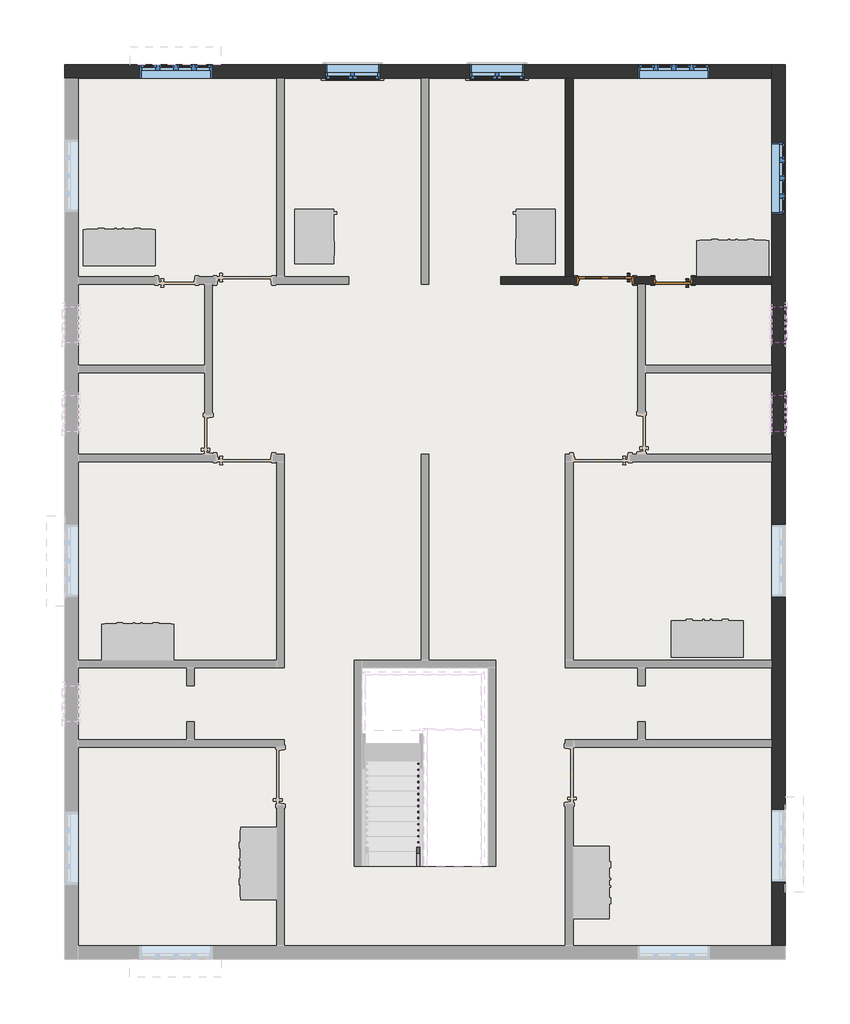
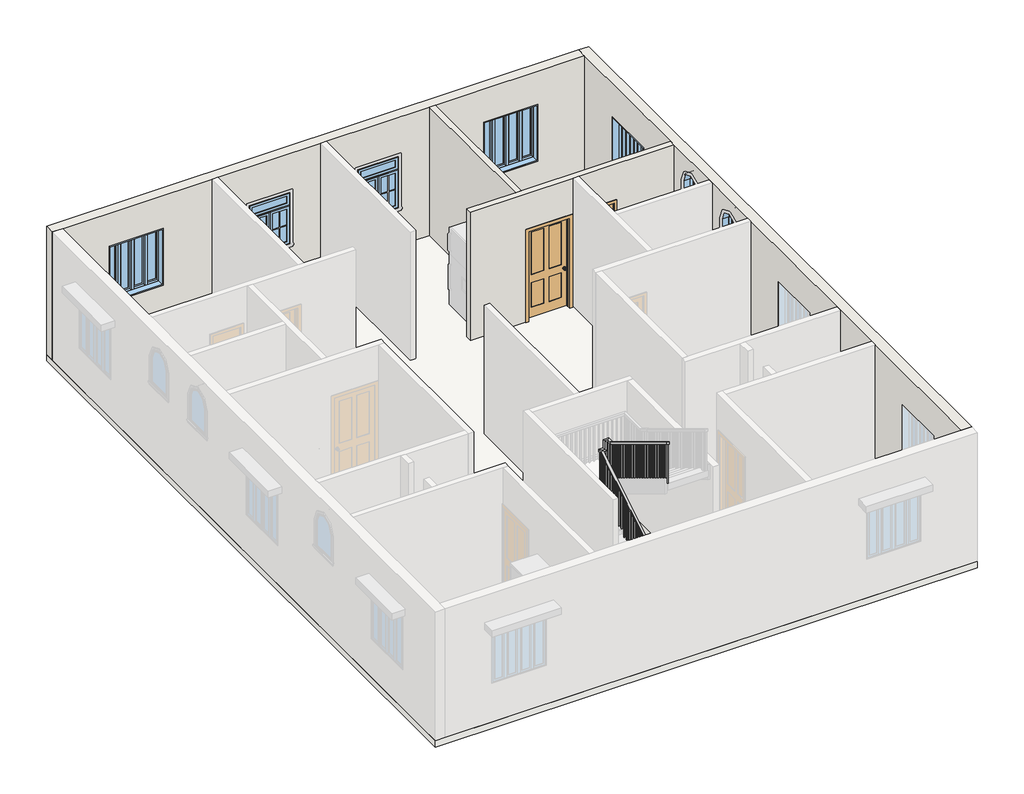
# One storey, part 2 of 4: 7 windows, 4 walls, 2 doors, 1 railing, 1 slab.
"""IFC4 building model written with IfcOpenShell, lengths in millimetres."""

from ifc_helpers import new_model, si_unit, frame, origin, place, context, project, spatial, polyline, circle_curve, outline, extrude, faceted_brep, transform, mapped, element, save
from ifc_brep_helpers import plane_surface, revolved_surface, advanced_brep
from components import door_a823658d, door_3f5f64ee, window_casement_double_transom_0fae6a54, window_casement_multi_sash_horizontal_main_windows_4_x_7_0e27d311, window_2fd4accf

model = new_model("IFC4")

# Units and contexts
model_context = context("Model", 3, world=origin())
ifc_project = project(units=[si_unit("LENGTHUNIT", "METRE", prefix="MILLI")], contexts=[model_context])

# Site, building, storey
site = spatial("IfcSite", under=ifc_project)
building = spatial("IfcBuilding", under=site)
storey = spatial("IfcBuildingStorey", under=building, Elevation=3352.8)

# Doors
placement = place(None, origin())
door_shape = door_a823658d(model_context)
element("IfcDoor", 1, ObjectType="Door-Interior-Single-4_Panel-Wood : 36\" x 84\"", at=placement, inside=storey, context=model_context, shape_type="MappedRepresentation", body=[
    mapped(door_shape, transform((-6490.9771954, 4939.0022103, 3352.8), x_axis=(-1.0, 0.0, 0.0), y_axis=(0.0, -1.0, 0.0), z_axis=(0.0, 0.0, 1.0))),
])
door_2_shape = door_3f5f64ee(model_context)
element("IfcDoor", 2, ObjectType="Door-Interior-Single-Flush_Panel-Wood : 24\" x 84\"", at=placement, inside=storey, context=model_context, shape_type="MappedRepresentation", body=[
    mapped(door_2_shape, transform((-5347.9771954, 4932.6522103, 3352.8), x_axis=(-1.0, 0.0, 0.0), y_axis=(0.0, -1.0, 0.0), z_axis=(0.0, 0.0, 1.0))),
])

# Railing
element("IfcRailing", 3, ObjectType="Handrail - Rectangular", at=placement, inside=storey, context=model_context, shape_type="SolidModel", body=[
    faceted_brep([(-9678.6771954, -4957.4727897, 4419.6), (-9678.6771954, -4957.4727897, 4360.3575287), (-9627.8771954, -4957.4727897, 4360.3575287), (-9627.8771954, -4957.4727897, 4419.6), (-9678.6771954, -2671.4727897, 5791.2), (-9678.6771954, -2657.4020042, 5740.4), (-9627.8771954, -2657.4020042, 5740.4), (-9627.8771954, -2671.4727897, 5791.2), (-9678.6771954, -2588.9227897, 5791.2), (-9678.6771954, -2588.9227897, 5740.4), (-9627.8771954, -2639.7227897, 5740.4), (-9627.8771954, -2639.7227897, 5791.2), (-9577.0771954, -2588.9227897, 5791.2), (-9526.2771954, -2588.9227897, 5740.4), (-9526.2771954, -2639.7227897, 5740.4), (-9577.0771954, -2639.7227897, 5791.2), (-9577.0771954, -2588.9227897, 5989.32), (-9526.2771954, -2588.9227897, 5938.52), (-9526.2771954, -2639.7227897, 5938.52), (-9577.0771954, -2639.7227897, 5989.32), (-9450.0771954, -2588.9227897, 5989.32), (-9450.0771954, -2588.9227897, 5938.52), (-9500.8771954, -2639.7227897, 5938.52), (-9500.8771954, -2639.7227897, 5989.32), (-9450.0771954, -2715.9227897, 5989.32), (-9450.0771954, -2729.9935751, 5938.52), (-9500.8771954, -2729.9935751, 5938.52), (-9500.8771954, -2715.9227897, 5989.32), (-9450.0771954, -4925.7227897, 7315.2), (-9500.8771954, -4925.7227897, 7315.2), (-9500.8771954, -4925.7227897, 7255.9575287), (-9450.0771954, -4925.7227897, 7255.9575287)], [[[0, 1, 2, 3]], [[1, 0, 4, 5]], [[2, 1, 5, 6]], [[3, 2, 6, 7]], [[0, 3, 7, 4]], [[5, 4, 8, 9]], [[6, 5, 9, 10]], [[7, 6, 10, 11]], [[4, 7, 11, 8]], [[9, 8, 12, 13]], [[10, 9, 13, 14]], [[11, 10, 14, 15]], [[8, 11, 15, 12]], [[13, 12, 16, 17]], [[14, 13, 17, 18]], [[15, 14, 18, 19]], [[12, 15, 19, 16]], [[17, 16, 20, 21]], [[18, 17, 21, 22]], [[19, 18, 22, 23]], [[16, 19, 23, 20]], [[21, 20, 24, 25]], [[22, 21, 25, 26]], [[23, 22, 26, 27]], [[20, 23, 27, 24]], [[28, 29, 30, 31]], [[25, 24, 28, 31]], [[26, 25, 31, 30]], [[27, 26, 30, 29]], [[24, 27, 29, 28]]]),
    extrude(outline(polyline([(-4859.0477897, 7215.9525287), (-4839.9977897, 7204.5225287), (-4839.9977897, 6248.4), (-4859.0477897, 6248.4), (-4859.0477897, 7215.9525287)])), frame((-9485.0021954, 0.0, 0.0), z_axis=(1.0, 0.0, 0.0), x_axis=(0.0, 1.0, 0.0)), (0.0, 0.0, 1.0), 19.05),
    extrude(outline(polyline([(-4757.4477897, 7154.9925287), (-4738.3977897, 7143.5625287), (-4738.3977897, 6248.4), (-4757.4477897, 6248.4), (-4757.4477897, 7154.9925287)])), frame((-9485.0021954, 0.0, 0.0), z_axis=(1.0, 0.0, 0.0), x_axis=(0.0, 1.0, 0.0)), (0.0, 0.0, 1.0), 19.05),
    extrude(outline(polyline([(-4655.8477897, 7094.0325287), (-4636.7977897, 7082.6025287), (-4636.7977897, 6096.0), (-4655.8477897, 6096.0), (-4655.8477897, 7094.0325287)])), frame((-9485.0021954, 0.0, 0.0), z_axis=(1.0, 0.0, 0.0), x_axis=(0.0, 1.0, 0.0)), (0.0, 0.0, 1.0), 19.05),
    extrude(outline(polyline([(-4554.2477897, 7033.0725287), (-4535.1977897, 7021.6425287), (-4535.1977897, 6096.0), (-4554.2477897, 6096.0), (-4554.2477897, 7033.0725287)])), frame((-9485.0021954, 0.0, 0.0), z_axis=(1.0, 0.0, 0.0), x_axis=(0.0, 1.0, 0.0)), (0.0, 0.0, 1.0), 19.05),
    extrude(outline(polyline([(-4452.6477897, 6972.1125287), (-4433.5977897, 6960.6825287), (-4433.5977897, 6096.0), (-4452.6477897, 6096.0), (-4452.6477897, 6972.1125287)])), frame((-9485.0021954, 0.0, 0.0), z_axis=(1.0, 0.0, 0.0), x_axis=(0.0, 1.0, 0.0)), (0.0, 0.0, 1.0), 19.05),
    extrude(outline(polyline([(-4351.0477897, 6911.1525287), (-4331.9977897, 6899.7225287), (-4331.9977897, 5943.6), (-4351.0477897, 5943.6), (-4351.0477897, 6911.1525287)])), frame((-9485.0021954, 0.0, 0.0), z_axis=(1.0, 0.0, 0.0), x_axis=(0.0, 1.0, 0.0)), (0.0, 0.0, 1.0), 19.05),
    extrude(outline(polyline([(-4249.4477897, 6850.1925287), (-4230.3977897, 6838.7625287), (-4230.3977897, 5943.6), (-4249.4477897, 5943.6), (-4249.4477897, 6850.1925287)])), frame((-9485.0021954, 0.0, 0.0), z_axis=(1.0, 0.0, 0.0), x_axis=(0.0, 1.0, 0.0)), (0.0, 0.0, 1.0), 19.05),
    extrude(outline(polyline([(-4147.8477897, 6789.2325287), (-4128.7977897, 6777.8025287), (-4128.7977897, 5791.2), (-4147.8477897, 5791.2), (-4147.8477897, 6789.2325287)])), frame((-9485.0021954, 0.0, 0.0), z_axis=(1.0, 0.0, 0.0), x_axis=(0.0, 1.0, 0.0)), (0.0, 0.0, 1.0), 19.05),
    extrude(outline(polyline([(-4046.2477897, 6728.2725287), (-4027.1977897, 6716.8425287), (-4027.1977897, 5791.2), (-4046.2477897, 5791.2), (-4046.2477897, 6728.2725287)])), frame((-9485.0021954, 0.0, 0.0), z_axis=(1.0, 0.0, 0.0), x_axis=(0.0, 1.0, 0.0)), (0.0, 0.0, 1.0), 19.05),
    extrude(outline(polyline([(-3944.6477897, 6667.3125287), (-3925.5977897, 6655.8825287), (-3925.5977897, 5791.2), (-3944.6477897, 5791.2), (-3944.6477897, 6667.3125287)])), frame((-9485.0021954, 0.0, 0.0), z_axis=(1.0, 0.0, 0.0), x_axis=(0.0, 1.0, 0.0)), (0.0, 0.0, 1.0), 19.05),
    extrude(outline(polyline([(-3843.0477897, 6606.3525287), (-3823.9977897, 6594.9225287), (-3823.9977897, 5638.8), (-3843.0477897, 5638.8), (-3843.0477897, 6606.3525287)])), frame((-9485.0021954, 0.0, 0.0), z_axis=(1.0, 0.0, 0.0), x_axis=(0.0, 1.0, 0.0)), (0.0, 0.0, 1.0), 19.05),
    extrude(outline(polyline([(-3741.4477897, 6545.3925287), (-3722.3977897, 6533.9625287), (-3722.3977897, 5638.8), (-3741.4477897, 5638.8), (-3741.4477897, 6545.3925287)])), frame((-9485.0021954, 0.0, 0.0), z_axis=(1.0, 0.0, 0.0), x_axis=(0.0, 1.0, 0.0)), (0.0, 0.0, 1.0), 19.05),
    extrude(outline(polyline([(-3639.8477897, 6484.4325287), (-3620.7977897, 6473.0025287), (-3620.7977897, 5486.4), (-3639.8477897, 5486.4), (-3639.8477897, 6484.4325287)])), frame((-9485.0021954, 0.0, 0.0), z_axis=(1.0, 0.0, 0.0), x_axis=(0.0, 1.0, 0.0)), (0.0, 0.0, 1.0), 19.05),
    extrude(outline(polyline([(-3538.2477897, 6423.4725287), (-3519.1977897, 6412.0425287), (-3519.1977897, 5486.4), (-3538.2477897, 5486.4), (-3538.2477897, 6423.4725287)])), frame((-9485.0021954, 0.0, 0.0), z_axis=(1.0, 0.0, 0.0), x_axis=(0.0, 1.0, 0.0)), (0.0, 0.0, 1.0), 19.05),
    extrude(outline(polyline([(-3436.6477897, 6362.5125287), (-3417.5977897, 6351.0825287), (-3417.5977897, 5486.4), (-3436.6477897, 5486.4), (-3436.6477897, 6362.5125287)])), frame((-9485.0021954, 0.0, 0.0), z_axis=(1.0, 0.0, 0.0), x_axis=(0.0, 1.0, 0.0)), (0.0, 0.0, 1.0), 19.05),
    extrude(outline(polyline([(-3335.0477897, 6301.5525287), (-3315.9977897, 6290.1225287), (-3315.9977897, 5334.0), (-3335.0477897, 5334.0), (-3335.0477897, 6301.5525287)])), frame((-9485.0021954, 0.0, 0.0), z_axis=(1.0, 0.0, 0.0), x_axis=(0.0, 1.0, 0.0)), (0.0, 0.0, 1.0), 19.05),
    extrude(outline(polyline([(-3233.4477897, 6240.5925287), (-3214.3977897, 6229.1625287), (-3214.3977897, 5334.0), (-3233.4477897, 5334.0), (-3233.4477897, 6240.5925287)])), frame((-9485.0021954, 0.0, 0.0), z_axis=(1.0, 0.0, 0.0), x_axis=(0.0, 1.0, 0.0)), (0.0, 0.0, 1.0), 19.05),
    extrude(outline(polyline([(-3131.8477897, 6179.6325287), (-3112.7977897, 6168.2025287), (-3112.7977897, 5181.6), (-3131.8477897, 5181.6), (-3131.8477897, 6179.6325287)])), frame((-9485.0021954, 0.0, 0.0), z_axis=(1.0, 0.0, 0.0), x_axis=(0.0, 1.0, 0.0)), (0.0, 0.0, 1.0), 19.05),
    extrude(outline(polyline([(-3030.2477897, 6118.6725287), (-3011.1977897, 6107.2425287), (-3011.1977897, 5181.6), (-3030.2477897, 5181.6), (-3030.2477897, 6118.6725287)])), frame((-9485.0021954, 0.0, 0.0), z_axis=(1.0, 0.0, 0.0), x_axis=(0.0, 1.0, 0.0)), (0.0, 0.0, 1.0), 19.05),
    extrude(outline(polyline([(-2928.6477897, 6057.7125287), (-2909.5977897, 6046.2825287), (-2909.5977897, 5181.6), (-2928.6477897, 5181.6), (-2928.6477897, 6057.7125287)])), frame((-9485.0021954, 0.0, 0.0), z_axis=(1.0, 0.0, 0.0), x_axis=(0.0, 1.0, 0.0)), (0.0, 0.0, 1.0), 19.05),
    extrude(outline(polyline([(-2827.0477897, 5996.7525287), (-2807.9977897, 5985.3225287), (-2807.9977897, 5029.2), (-2827.0477897, 5029.2), (-2827.0477897, 5996.7525287)])), frame((-9485.0021954, 0.0, 0.0), z_axis=(1.0, 0.0, 0.0), x_axis=(0.0, 1.0, 0.0)), (0.0, 0.0, 1.0), 19.05),
    extrude(outline(polyline([(-2725.4477897, 5935.7925287), (-2706.3977897, 5924.3625287), (-2706.3977897, 5029.2), (-2725.4477897, 5029.2), (-2725.4477897, 5935.7925287)])), frame((-9485.0021954, 0.0, 0.0), z_axis=(1.0, 0.0, 0.0), x_axis=(0.0, 1.0, 0.0)), (0.0, 0.0, 1.0), 19.05),
    extrude(outline(polyline([(-9561.2021954, -2623.8477897), (-9561.2021954, -2604.7977897), (-9542.1521954, -2604.7977897), (-9542.1521954, -2623.8477897), (-9561.2021954, -2623.8477897)])), frame((0.0, 0.0, 4876.8), z_axis=(0.0, 0.0, 1.0), x_axis=(1.0, 0.0, 0.0)), (0.0, 0.0, 1.0), 1061.72),
    extrude(outline(polyline([(-2731.7977897, 5695.7625287), (-2712.7477897, 5707.1925287), (-2712.7477897, 4724.4), (-2731.7977897, 4724.4), (-2731.7977897, 5695.7625287)])), frame((-9662.8021954, 0.0, 0.0), z_axis=(1.0, 0.0, 0.0), x_axis=(0.0, 1.0, 0.0)), (0.0, 0.0, 1.0), 19.05),
    extrude(outline(polyline([(-2833.3977897, 5634.8025287), (-2814.3477897, 5646.2325287), (-2814.3477897, 4724.4), (-2833.3977897, 4724.4), (-2833.3977897, 5634.8025287)])), frame((-9662.8021954, 0.0, 0.0), z_axis=(1.0, 0.0, 0.0), x_axis=(0.0, 1.0, 0.0)), (0.0, 0.0, 1.0), 19.05),
    extrude(outline(polyline([(-2934.9977897, 5573.8425287), (-2915.9477897, 5585.2725287), (-2915.9477897, 4724.4), (-2934.9977897, 4724.4), (-2934.9977897, 5573.8425287)])), frame((-9662.8021954, 0.0, 0.0), z_axis=(1.0, 0.0, 0.0), x_axis=(0.0, 1.0, 0.0)), (0.0, 0.0, 1.0), 19.05),
    extrude(outline(polyline([(-3036.5977897, 5512.8825287), (-3017.5477897, 5524.3125287), (-3017.5477897, 4572.0), (-3036.5977897, 4572.0), (-3036.5977897, 5512.8825287)])), frame((-9662.8021954, 0.0, 0.0), z_axis=(1.0, 0.0, 0.0), x_axis=(0.0, 1.0, 0.0)), (0.0, 0.0, 1.0), 19.05),
    extrude(outline(polyline([(-3138.1977897, 5451.9225287), (-3119.1477897, 5463.3525287), (-3119.1477897, 4572.0), (-3138.1977897, 4572.0), (-3138.1977897, 5451.9225287)])), frame((-9662.8021954, 0.0, 0.0), z_axis=(1.0, 0.0, 0.0), x_axis=(0.0, 1.0, 0.0)), (0.0, 0.0, 1.0), 19.05),
    extrude(outline(polyline([(-3239.7977897, 5390.9625287), (-3220.7477897, 5402.3925287), (-3220.7477897, 4419.6), (-3239.7977897, 4419.6), (-3239.7977897, 5390.9625287)])), frame((-9662.8021954, 0.0, 0.0), z_axis=(1.0, 0.0, 0.0), x_axis=(0.0, 1.0, 0.0)), (0.0, 0.0, 1.0), 19.05),
    extrude(outline(polyline([(-3341.3977897, 5330.0025287), (-3322.3477897, 5341.4325287), (-3322.3477897, 4419.6), (-3341.3977897, 4419.6), (-3341.3977897, 5330.0025287)])), frame((-9662.8021954, 0.0, 0.0), z_axis=(1.0, 0.0, 0.0), x_axis=(0.0, 1.0, 0.0)), (0.0, 0.0, 1.0), 19.05),
    extrude(outline(polyline([(-3442.9977897, 5269.0425287), (-3423.9477897, 5280.4725287), (-3423.9477897, 4419.6), (-3442.9977897, 4419.6), (-3442.9977897, 5269.0425287)])), frame((-9662.8021954, 0.0, 0.0), z_axis=(1.0, 0.0, 0.0), x_axis=(0.0, 1.0, 0.0)), (0.0, 0.0, 1.0), 19.05),
    extrude(outline(polyline([(-3544.5977897, 5208.0825287), (-3525.5477897, 5219.5125287), (-3525.5477897, 4267.2), (-3544.5977897, 4267.2), (-3544.5977897, 5208.0825287)])), frame((-9662.8021954, 0.0, 0.0), z_axis=(1.0, 0.0, 0.0), x_axis=(0.0, 1.0, 0.0)), (0.0, 0.0, 1.0), 19.05),
    extrude(outline(polyline([(-3646.1977897, 5147.1225287), (-3627.1477897, 5158.5525287), (-3627.1477897, 4267.2), (-3646.1977897, 4267.2), (-3646.1977897, 5147.1225287)])), frame((-9662.8021954, 0.0, 0.0), z_axis=(1.0, 0.0, 0.0), x_axis=(0.0, 1.0, 0.0)), (0.0, 0.0, 1.0), 19.05),
    extrude(outline(polyline([(-3747.7977897, 5086.1625287), (-3728.7477897, 5097.5925287), (-3728.7477897, 4114.8), (-3747.7977897, 4114.8), (-3747.7977897, 5086.1625287)])), frame((-9662.8021954, 0.0, 0.0), z_axis=(1.0, 0.0, 0.0), x_axis=(0.0, 1.0, 0.0)), (0.0, 0.0, 1.0), 19.05),
    extrude(outline(polyline([(-3849.3977897, 5025.2025287), (-3830.3477897, 5036.6325287), (-3830.3477897, 4114.8), (-3849.3977897, 4114.8), (-3849.3977897, 5025.2025287)])), frame((-9662.8021954, 0.0, 0.0), z_axis=(1.0, 0.0, 0.0), x_axis=(0.0, 1.0, 0.0)), (0.0, 0.0, 1.0), 19.05),
    extrude(outline(polyline([(-3950.9977897, 4964.2425287), (-3931.9477897, 4975.6725287), (-3931.9477897, 4114.8), (-3950.9977897, 4114.8), (-3950.9977897, 4964.2425287)])), frame((-9662.8021954, 0.0, 0.0), z_axis=(1.0, 0.0, 0.0), x_axis=(0.0, 1.0, 0.0)), (0.0, 0.0, 1.0), 19.05),
    extrude(outline(polyline([(-4052.5977897, 4903.2825287), (-4033.5477897, 4914.7125287), (-4033.5477897, 3962.4), (-4052.5977897, 3962.4), (-4052.5977897, 4903.2825287)])), frame((-9662.8021954, 0.0, 0.0), z_axis=(1.0, 0.0, 0.0), x_axis=(0.0, 1.0, 0.0)), (0.0, 0.0, 1.0), 19.05),
    extrude(outline(polyline([(-4154.1977897, 4842.3225287), (-4135.1477897, 4853.7525287), (-4135.1477897, 3962.4), (-4154.1977897, 3962.4), (-4154.1977897, 4842.3225287)])), frame((-9662.8021954, 0.0, 0.0), z_axis=(1.0, 0.0, 0.0), x_axis=(0.0, 1.0, 0.0)), (0.0, 0.0, 1.0), 19.05),
    extrude(outline(polyline([(-4255.7977897, 4781.3625287), (-4236.7477897, 4792.7925287), (-4236.7477897, 3810.0), (-4255.7977897, 3810.0), (-4255.7977897, 4781.3625287)])), frame((-9662.8021954, 0.0, 0.0), z_axis=(1.0, 0.0, 0.0), x_axis=(0.0, 1.0, 0.0)), (0.0, 0.0, 1.0), 19.05),
    extrude(outline(polyline([(-4357.3977897, 4720.4025287), (-4338.3477897, 4731.8325287), (-4338.3477897, 3810.0), (-4357.3977897, 3810.0), (-4357.3977897, 4720.4025287)])), frame((-9662.8021954, 0.0, 0.0), z_axis=(1.0, 0.0, 0.0), x_axis=(0.0, 1.0, 0.0)), (0.0, 0.0, 1.0), 19.05),
    extrude(outline(polyline([(-4458.9977897, 4659.4425287), (-4439.9477897, 4670.8725287), (-4439.9477897, 3810.0), (-4458.9977897, 3810.0), (-4458.9977897, 4659.4425287)])), frame((-9662.8021954, 0.0, 0.0), z_axis=(1.0, 0.0, 0.0), x_axis=(0.0, 1.0, 0.0)), (0.0, 0.0, 1.0), 19.05),
    extrude(outline(polyline([(-4560.5977897, 4598.4825287), (-4541.5477897, 4609.9125287), (-4541.5477897, 3657.6), (-4560.5977897, 3657.6), (-4560.5977897, 4598.4825287)])), frame((-9662.8021954, 0.0, 0.0), z_axis=(1.0, 0.0, 0.0), x_axis=(0.0, 1.0, 0.0)), (0.0, 0.0, 1.0), 19.05),
    extrude(outline(polyline([(-4662.1977897, 4537.5225287), (-4643.1477897, 4548.9525287), (-4643.1477897, 3657.6), (-4662.1977897, 3657.6), (-4662.1977897, 4537.5225287)])), frame((-9662.8021954, 0.0, 0.0), z_axis=(1.0, 0.0, 0.0), x_axis=(0.0, 1.0, 0.0)), (0.0, 0.0, 1.0), 19.05),
    extrude(outline(polyline([(-4763.7977897, 4476.5625287), (-4744.7477897, 4487.9925287), (-4744.7477897, 3505.2), (-4763.7977897, 3505.2), (-4763.7977897, 4476.5625287)])), frame((-9662.8021954, 0.0, 0.0), z_axis=(1.0, 0.0, 0.0), x_axis=(0.0, 1.0, 0.0)), (0.0, 0.0, 1.0), 19.05),
    extrude(outline(polyline([(-4865.3977897, 4415.6025287), (-4846.3477897, 4427.0325287), (-4846.3477897, 3505.2), (-4865.3977897, 3505.2), (-4865.3977897, 4415.6025287)])), frame((-9662.8021954, 0.0, 0.0), z_axis=(1.0, 0.0, 0.0), x_axis=(0.0, 1.0, 0.0)), (0.0, 0.0, 1.0), 19.05),
    extrude(outline(polyline([(-9485.0021954, -2623.8477897), (-9485.0021954, -2604.7977897), (-9465.9521954, -2604.7977897), (-9465.9521954, -2623.8477897), (-9485.0021954, -2623.8477897)])), frame((0.0, 0.0, 4876.8), z_axis=(0.0, 0.0, 1.0), x_axis=(1.0, 0.0, 0.0)), (0.0, 0.0, 1.0), 1061.72),
    extrude(outline(polyline([(-9643.7521954, -2623.8477897), (-9662.8021954, -2623.8477897), (-9662.8021954, -2604.7977897), (-9643.7521954, -2604.7977897), (-9643.7521954, -2623.8477897)])), frame((0.0, 0.0, 4876.8), z_axis=(0.0, 0.0, 1.0), x_axis=(1.0, 0.0, 0.0)), (0.0, 0.0, 1.0), 863.6),
    extrude(outline(polyline([(-2680.9977897, 5726.2425287), (-2661.9477897, 5737.6725287), (-2661.9477897, 4876.8), (-2680.9977897, 4876.8), (-2680.9977897, 5726.2425287)])), frame((-9662.8021954, 0.0, 0.0), z_axis=(1.0, 0.0, 0.0), x_axis=(0.0, 1.0, 0.0)), (0.0, 0.0, 1.0), 19.05),
    extrude(outline(polyline([(-4925.7227897, 7255.9575287), (-4906.6727897, 7244.5275287), (-4906.6727897, 6248.4), (-4925.7227897, 6248.4), (-4925.7227897, 7255.9575287)])), frame((-9485.0021954, 0.0, 0.0), z_axis=(1.0, 0.0, 0.0), x_axis=(0.0, 1.0, 0.0)), (0.0, 0.0, 1.0), 19.05),
    extrude(outline(polyline([(-4957.4727897, 4360.3575287), (-4938.4227897, 4371.7875287), (-4938.4227897, 3505.2), (-4957.4727897, 3505.2), (-4957.4727897, 4360.3575287)])), frame((-9662.8021954, 0.0, 0.0), z_axis=(1.0, 0.0, 0.0), x_axis=(0.0, 1.0, 0.0)), (0.0, 0.0, 1.0), 19.05),
])

# Slab
element("IfcSlab", 4, ObjectType="MARBLE FLOORING 6\"", at=placement, inside=storey, context=model_context, shape_type="SweptSolid", body=[
    extrude(outline(polyline([(-3455.6771954, 8580.7272103), (-3455.6771954, -6532.2727897), (-15623.8646954, -6532.2727897), (-15623.8646954, 8580.7272103), (-3455.6771954, 8580.7272103)]), holes=[polyline([(-10605.7771954, -4957.4727897), (-8472.1771954, -4957.4727897), (-8472.1771954, -1604.6727897), (-10605.7771954, -1604.6727897), (-10605.7771954, -4957.4727897)])]), frame((0.0, 0.0, 3200.4), z_axis=(0.0, 0.0, 1.0), x_axis=(1.0, 0.0, 0.0)), (0.0, 0.0, 1.0), 152.4),
])

# Walls
element("IfcWall", 5, ObjectType="INNER WALL 5\"", at=placement, inside=storey, context=model_context, shape_type="Brep", body=[
    faceted_brep([(-3684.2771954, 4872.3272103, 6400.8), (-5817.8771954, 4872.3272103, 6400.8), (-5944.8771954, 4872.3272103, 6400.8), (-8256.2771954, 4872.3272103, 6400.8), (-8256.2771954, 4872.3272103, 3352.8), (-6973.5771954, 4872.3272103, 3352.8), (-6973.5771954, 4872.3272103, 5511.8), (-6008.3771954, 4872.3272103, 5511.8), (-6008.3771954, 4872.3272103, 3352.8), (-5944.8771954, 4872.3272103, 3352.8), (-5817.8771954, 4872.3272103, 3352.8), (-5678.1771954, 4872.3272103, 3352.8), (-5678.1771954, 4872.3272103, 5511.8), (-5017.7771954, 4872.3272103, 5511.8), (-5017.7771954, 4872.3272103, 3352.8), (-3684.2771954, 4872.3272103, 3352.8), (-8256.2771954, 4999.3272103, 6400.8), (-7164.0771954, 4999.3272103, 6400.8), (-7037.0771954, 4999.3272103, 6400.8), (-3684.2771954, 4999.3272103, 6400.8), (-3684.2771954, 4999.3272103, 3352.8), (-5017.7771954, 4999.3272103, 3352.8), (-5017.7771954, 4999.3272103, 5511.8), (-5678.1771954, 4999.3272103, 5511.8), (-5678.1771954, 4999.3272103, 3352.8), (-6008.3771954, 4999.3272103, 3352.8), (-6008.3771954, 4999.3272103, 5511.8), (-6973.5771954, 4999.3272103, 5511.8), (-6973.5771954, 4999.3272103, 3352.8), (-7037.0771954, 4999.3272103, 3352.8), (-7164.0771954, 4999.3272103, 3352.8), (-8256.2771954, 4999.3272103, 3352.8)], [[[0, 1, 2, 3, 4, 5, 6, 7, 8, 9, 10, 11, 12, 13, 14, 15]], [[16, 17, 18, 19, 20, 21, 22, 23, 24, 25, 26, 27, 28, 29, 30, 31]], [[4, 31, 30, 29, 28, 5]], [[20, 15, 14, 21]], [[8, 25, 24, 11, 10, 9]], [[3, 2, 1, 0, 19, 18, 17, 16]], [[4, 3, 16, 31]], [[0, 15, 20, 19]], [[27, 6, 5, 28]], [[6, 27, 26, 7]], [[7, 26, 25, 8]], [[23, 12, 11, 24]], [[12, 23, 22, 13]], [[13, 22, 21, 14]]]),
])
element("IfcWall", 6, ObjectType="INNER WALL 5\"", at=placement, inside=storey, context=model_context, shape_type="SweptSolid", body=[
    extrude(outline(polyline([(-7164.0771954, 4999.3272103), (-7164.0771954, 8352.1272103), (-7037.0771954, 8352.1272103), (-7037.0771954, 4999.3272103), (-7164.0771954, 4999.3272103)])), frame((0.0, 0.0, 3352.8), z_axis=(0.0, 0.0, 1.0), x_axis=(1.0, 0.0, 0.0)), (0.0, 0.0, 1.0), 3048.0),
])
element("IfcWall", 7, ObjectType="OUTER WALL 9\"", at=placement, inside=storey, context=model_context, shape_type="Brep", body=[
    faceted_brep([(-15623.8646954, 8352.1272103, 3352.8), (-15395.2646954, 8352.1272103, 3352.8), (-12040.8771954, 8352.1272103, 3352.8), (-11913.8771954, 8352.1272103, 3352.8), (-9602.4771954, 8352.1272103, 3352.8), (-9475.4771954, 8352.1272103, 3352.8), (-7164.0771954, 8352.1272103, 3352.8), (-7037.0771954, 8352.1272103, 3352.8), (-3684.2771954, 8352.1272103, 3352.8), (-3684.2771954, 8352.1272103, 6400.8), (-7037.0771954, 8352.1272103, 6400.8), (-7164.0771954, 8352.1272103, 6400.8), (-9475.4771954, 8352.1272103, 6400.8), (-9602.4771954, 8352.1272103, 6400.8), (-11913.8771954, 8352.1272103, 6400.8), (-12040.8771954, 8352.1272103, 6400.8), (-15395.2646954, 8352.1272103, 6400.8), (-15623.8646954, 8352.1272103, 6400.8), (-13133.8709454, 8352.1272103, 5613.4), (-13133.8709454, 8352.1272103, 4267.2), (-14353.0709454, 8352.1272103, 4267.2), (-14353.0709454, 8352.1272103, 5613.4), (-4725.6771954, 8352.1272103, 5613.4), (-4725.6771954, 8352.1272103, 4267.2), (-5944.8771954, 8352.1272103, 4267.2), (-5944.8771954, 8352.1272103, 5613.4), (-10300.9771954, 8352.1272103, 5486.4), (-10300.9771954, 8352.1272103, 4267.2), (-11215.3771954, 8352.1272103, 4267.2), (-11215.3771954, 8352.1272103, 5486.4), (-7862.5771954, 8352.1272103, 5486.4), (-7862.5771954, 8352.1272103, 4267.2), (-8776.9771954, 8352.1272103, 4267.2), (-8776.9771954, 8352.1272103, 5486.4), (-15623.8646954, 8580.7272103, 3352.8), (-15623.8646954, 8580.7272103, 6400.8), (-3684.2771954, 8580.7272103, 6400.8), (-3684.2771954, 8580.7272103, 3352.8), (-13133.8709454, 8580.7272103, 5613.4), (-14353.0709454, 8580.7272103, 5613.4), (-14353.0709454, 8580.7272103, 4267.2), (-13133.8709454, 8580.7272103, 4267.2), (-4725.6771954, 8580.7272103, 5613.4), (-5944.8771954, 8580.7272103, 5613.4), (-5944.8771954, 8580.7272103, 4267.2), (-4725.6771954, 8580.7272103, 4267.2), (-10300.9771954, 8580.7272103, 5486.4), (-11215.3771954, 8580.7272103, 5486.4), (-11215.3771954, 8580.7272103, 4267.2), (-10300.9771954, 8580.7272103, 4267.2), (-7862.5771954, 8580.7272103, 5486.4), (-8776.9771954, 8580.7272103, 5486.4), (-8776.9771954, 8580.7272103, 4267.2), (-7862.5771954, 8580.7272103, 4267.2)], [[[0, 1, 2, 3, 4, 5, 6, 7, 8, 9, 10, 11, 12, 13, 14, 15, 16, 17], [18, 19, 20, 21], [22, 23, 24, 25], [26, 27, 28, 29], [30, 31, 32, 33]], [[34, 35, 36, 37], [38, 39, 40, 41], [42, 43, 44, 45], [46, 47, 48, 49], [50, 51, 52, 53]], [[8, 7, 6, 5, 4, 3, 2, 1, 0, 34, 37]], [[17, 16, 15, 14, 13, 12, 11, 10, 9, 36, 35]], [[0, 17, 35, 34]], [[9, 8, 37, 36]], [[19, 18, 38, 41]], [[20, 19, 41, 40]], [[21, 20, 40, 39]], [[18, 21, 39, 38]], [[23, 22, 42, 45]], [[24, 23, 45, 44]], [[25, 24, 44, 43]], [[22, 25, 43, 42]], [[27, 26, 46, 49]], [[28, 27, 49, 48]], [[29, 28, 48, 47]], [[26, 29, 47, 46]], [[31, 30, 50, 53]], [[32, 31, 53, 52]], [[33, 32, 52, 51]], [[30, 33, 51, 50]]]),
])
element("IfcWall", 8, ObjectType="OUTER WALL 9\"", at=placement, inside=storey, context=model_context, shape_type="AdvancedBrep", body=[
    advanced_brep(
    [(-3684.2771954, 8580.7272103, 3352.8), (-3684.2771954, 8352.1272103, 3352.8), (-3684.2771954, 4999.3272103, 3352.8), (-3684.2771954, 4872.3272103, 3352.8), (-3684.2771954, 3500.7272103, 3352.8), (-3684.2771954, 3373.7272103, 3352.8), (-3684.2771954, 2002.6566069, 3352.8), (-3684.2771954, 1875.6566069, 3352.8), (-3684.2771954, -1477.6727897, 3352.8), (-3684.2771954, -1604.6727897, 3352.8), (-3684.2771954, -2823.8727897, 3352.8), (-3684.2771954, -2950.8727897, 3352.8), (-3684.2771954, -6303.6727897, 3352.8), (-3684.2771954, -6303.6727897, 6400.8), (-3684.2771954, -2950.8727897, 6400.8), (-3684.2771954, -2823.8727897, 6400.8), (-3684.2771954, -1604.6727897, 6400.8), (-3684.2771954, -1477.6727897, 6400.8), (-3684.2771954, 1875.6566069, 6400.8), (-3684.2771954, 2002.6566069, 6400.8), (-3684.2771954, 3373.7272103, 6400.8), (-3684.2771954, 3500.7272103, 6400.8), (-3684.2771954, 4872.3272103, 6400.8), (-3684.2771954, 4999.3272103, 6400.8), (-3684.2771954, 8352.1272103, 6400.8), (-3684.2771954, 8580.7272103, 6400.8), (-3684.2771954, 6053.4272103, 5613.4), (-3684.2771954, 6053.4272103, 4267.2), (-3684.2771954, 7272.6272103, 4267.2), (-3684.2771954, 7272.6272103, 5613.4), (-3684.2771954, -410.6080914, 5613.4), (-3684.2771954, -410.6080914, 4267.2), (-3684.2771954, 808.5919086, 4267.2), (-3684.2771954, 808.5919086, 5613.4), (-3684.2771954, -4004.9727897, 5613.4), (-3684.2771954, -5224.1727897, 5613.4), (-3684.2771954, -5224.1727897, 4267.2), (-3684.2771954, -4004.9727897, 4267.2), (-3684.2771954, 2992.9919086, 5181.6), (-3684.2771954, 2992.9919086, 5791.2), (-3684.2771954, 2383.3919086, 5791.2), (-3684.2771954, 2383.3919086, 5181.6), (-3684.2771954, 4491.3272103, 5181.6), (-3684.2771954, 4491.3272103, 5791.2), (-3684.2771954, 3881.7272103, 5791.2), (-3684.2771954, 3881.7272103, 5181.6), (-3455.6771954, 8580.7272103, 3352.8), (-3455.6771954, 8580.7272103, 6400.8), (-3455.6771954, -6303.6727897, 6400.8), (-3455.6771954, -6303.6727897, 3352.8), (-3455.6771954, 6053.4272103, 5613.4), (-3455.6771954, 7272.6272103, 5613.4), (-3455.6771954, 7272.6272103, 4267.2), (-3455.6771954, 6053.4272103, 4267.2), (-3455.6771954, -410.6080914, 5613.4), (-3455.6771954, 808.5919086, 5613.4), (-3455.6771954, 808.5919086, 4267.2), (-3455.6771954, -410.6080914, 4267.2), (-3455.6771954, -4004.9727897, 5613.4), (-3455.6771954, -4004.9727897, 4267.2), (-3455.6771954, -5224.1727897, 4267.2), (-3455.6771954, -5224.1727897, 5613.4), (-3455.6771954, 2992.9919086, 5181.6), (-3455.6771954, 2383.3919086, 5181.6), (-3455.6771954, 2383.3919086, 5791.2), (-3455.6771954, 2992.9919086, 5791.2), (-3455.6771954, 4491.3272103, 5181.6), (-3455.6771954, 3881.7272103, 5181.6), (-3455.6771954, 3881.7272103, 5791.2), (-3455.6771954, 4491.3272103, 5791.2)],
    [
        (0, 1),
        (1, 2),
        (2, 3),
        (3, 4),
        (4, 5),
        (5, 6),
        (6, 7),
        (7, 8),
        (8, 9),
        (9, 10),
        (10, 11),
        (11, 12),
        (12, 13),
        (13, 14),
        (14, 15),
        (15, 16),
        (16, 17),
        (17, 18),
        (18, 19),
        (19, 20),
        (20, 21),
        (21, 22),
        (22, 23),
        (23, 24),
        (24, 25),
        (25, 0),
        (26, 27),
        (27, 28),
        (28, 29),
        (29, 26),
        (30, 31),
        (31, 32),
        (32, 33),
        (33, 30),
        (34, 35),
        (35, 36),
        (36, 37),
        (37, 34),
        (38, 39),
        (39, 40, circle_curve(frame((-3684.2771954, 2688.1919086, 5791.2), z_axis=(1.0, 0.0, 0.0), x_axis=(0.0, -1.0, 0.0)), 304.8)),
        (40, 41),
        (41, 38),
        (42, 43),
        (43, 44, circle_curve(frame((-3684.2771954, 4186.5272103, 5791.2), z_axis=(1.0, 0.0, 0.0), x_axis=(0.0, -1.0, 0.0)), 304.8)),
        (44, 45),
        (45, 42),
        (46, 47),
        (47, 48),
        (48, 49),
        (49, 46),
        (50, 51),
        (51, 52),
        (52, 53),
        (53, 50),
        (54, 55),
        (55, 56),
        (56, 57),
        (57, 54),
        (58, 59),
        (59, 60),
        (60, 61),
        (61, 58),
        (62, 63),
        (63, 64),
        (64, 65, circle_curve(frame((-3455.6771954, 2688.1919086, 5791.2), z_axis=(-1.0, 0.0, 0.0), x_axis=(0.0, -1.0, 0.0)), 304.8)),
        (65, 62),
        (66, 67),
        (67, 68),
        (68, 69, circle_curve(frame((-3455.6771954, 4186.5272103, 5791.2), z_axis=(-1.0, 0.0, 0.0), x_axis=(0.0, -1.0, 0.0)), 304.8)),
        (69, 66),
        (0, 46),
        (49, 12),
        (13, 48),
        (47, 25),
        (26, 50),
        (53, 27),
        (52, 28),
        (51, 29),
        (30, 54),
        (57, 31),
        (56, 32),
        (55, 33),
        (58, 34),
        (37, 59),
        (36, 60),
        (35, 61),
        (62, 38),
        (41, 63),
        (40, 64),
        (39, 65),
        (66, 42),
        (45, 67),
        (44, 68),
        (43, 69),
    ],
    [
        plane_surface(frame((-3684.2771954, 8466.4272103, 3352.8), z_axis=(-1.0, 0.0, 0.0), x_axis=(0.0, -1.0, 0.0))),
        plane_surface(frame((-3455.6771954, 8466.4272103, 3352.8), z_axis=(1.0, 0.0, 0.0), x_axis=(0.0, 1.0, 0.0))),
        plane_surface(frame((-3684.2771954, 8466.4272103, 3352.8), z_axis=(0.0, 0.0, -1.0), x_axis=(1.0, 0.0, 0.0))),
        plane_surface(frame((-3684.2771954, -6417.9727897, 6400.8), z_axis=(0.0, 0.0, 1.0), x_axis=(1.0, 0.0, 0.0))),
        plane_surface(frame((-15509.5646954, 8580.7272103, 3352.8), z_axis=(0.0, 1.0, 0.0), x_axis=(-1.0, 0.0, 0.0))),
        plane_surface(frame((-3569.9771954, -6303.6727897, 3352.8), z_axis=(0.0, -1.0, 0.0), x_axis=(-1.0, 0.0, 0.0))),
        plane_surface(frame((-3684.2771954, 6053.4272103, 5613.4), z_axis=(0.0, 1.0, 0.0), x_axis=(1.0, 0.0, 0.0))),
        plane_surface(frame((-3684.2771954, 6053.4272103, 4267.2), z_axis=(0.0, 0.0, 1.0), x_axis=(1.0, 0.0, 0.0))),
        plane_surface(frame((-3684.2771954, 7272.6272103, 4267.2), z_axis=(0.0, -1.0, 0.0), x_axis=(1.0, 0.0, 0.0))),
        plane_surface(frame((-3684.2771954, 7272.6272103, 5613.4), z_axis=(0.0, 0.0, -1.0), x_axis=(1.0, 0.0, 0.0))),
        plane_surface(frame((-3684.2771954, -410.6080914, 5613.4), z_axis=(0.0, 1.0, 0.0), x_axis=(1.0, 0.0, 0.0))),
        plane_surface(frame((-3684.2771954, -410.6080914, 4267.2), z_axis=(0.0, 0.0, 1.0), x_axis=(1.0, 0.0, 0.0))),
        plane_surface(frame((-3684.2771954, 808.5919086, 4267.2), z_axis=(0.0, -1.0, 0.0), x_axis=(1.0, 0.0, 0.0))),
        plane_surface(frame((-3684.2771954, 808.5919086, 5613.4), z_axis=(0.0, 0.0, -1.0), x_axis=(1.0, 0.0, 0.0))),
        plane_surface(frame((-3455.6771954, -4004.9727897, 5613.4), z_axis=(0.0, -1.0, 0.0), x_axis=(-1.0, 0.0, 0.0))),
        plane_surface(frame((-3455.6771954, -4004.9727897, 4267.2), z_axis=(0.0, 0.0, 1.0), x_axis=(-1.0, 0.0, 0.0))),
        plane_surface(frame((-3455.6771954, -5224.1727897, 4267.2), z_axis=(0.0, 1.0, 0.0), x_axis=(-1.0, 0.0, 0.0))),
        plane_surface(frame((-3455.6771954, -5224.1727897, 5613.4), z_axis=(0.0, 0.0, -1.0), x_axis=(-1.0, 0.0, 0.0))),
        plane_surface(frame((-3455.6771954, 2992.9919086, 5181.6), z_axis=(0.0, 0.0, 1.0), x_axis=(-1.0, 0.0, 0.0))),
        plane_surface(frame((-3455.6771954, 2383.3919086, 5181.6), z_axis=(0.0, 1.0, 0.0), x_axis=(-1.0, 0.0, 0.0))),
        revolved_surface(polyline([(-3684.2771954, 2383.3919085999996, 5791.2), (-3455.6771954, 2383.3919085999996, 5791.2)]), (-3684.2771954, 2688.1919086, 5791.2), (-1.0, 0.0, 0.0)),
        plane_surface(frame((-3455.6771954, 2992.9919086, 5791.2), z_axis=(0.0, -1.0, 0.0), x_axis=(-1.0, 0.0, 0.0))),
        plane_surface(frame((-3455.6771954, 4491.3272103, 5181.6), z_axis=(0.0, 0.0, 1.0), x_axis=(-1.0, 0.0, 0.0))),
        plane_surface(frame((-3455.6771954, 3881.7272103, 5181.6), z_axis=(0.0, 1.0, 0.0), x_axis=(-1.0, 0.0, 0.0))),
        revolved_surface(polyline([(-3684.2771954, 3881.7272102999996, 5791.2), (-3455.6771954, 3881.7272102999996, 5791.2)]), (-3684.2771954, 4186.5272103, 5791.2), (-1.0, 0.0, 0.0)),
        plane_surface(frame((-3455.6771954, 4491.3272103, 5791.2), z_axis=(0.0, -1.0, 0.0), x_axis=(-1.0, 0.0, 0.0))),
    ],
    [
        (0, [[1, 2, 3, 4, 5, 6, 7, 8, 9, 10, 11, 12, 13, 14, 15, 16, 17, 18, 19, 20, 21, 22, 23, 24, 25, 26], [27, 28, 29, 30], [31, 32, 33, 34], [35, 36, 37, 38], [39, 40, 41, 42], [43, 44, 45, 46]]),
        (1, [[47, 48, 49, 50], [51, 52, 53, 54], [55, 56, 57, 58], [59, 60, 61, 62], [63, 64, 65, 66], [67, 68, 69, 70]]),
        (2, [[-12, -11, -10, -9, -8, -7, -6, -5, -4, -3, -2, -1, 71, -50, 72]]),
        (3, [[-25, -24, -23, -22, -21, -20, -19, -18, -17, -16, -15, -14, 73, -48, 74]]),
        (4, [[-26, -74, -47, -71]]),
        (5, [[-13, -72, -49, -73]]),
        (6, [[-27, 75, -54, 76]]),
        (7, [[-28, -76, -53, 77]]),
        (8, [[-29, -77, -52, 78]]),
        (9, [[-30, -78, -51, -75]]),
        (10, [[-31, 79, -58, 80]]),
        (11, [[-32, -80, -57, 81]]),
        (12, [[-33, -81, -56, 82]]),
        (13, [[-34, -82, -55, -79]]),
        (14, [[-59, 83, -38, 84]]),
        (15, [[-60, -84, -37, 85]]),
        (16, [[-61, -85, -36, 86]]),
        (17, [[-62, -86, -35, -83]]),
        (18, [[-63, 87, -42, 88]]),
        (19, [[-64, -88, -41, 89]]),
        (20, [[-65, -89, -40, 90]]),
        (21, [[-66, -90, -39, -87]]),
        (22, [[-67, 91, -46, 92]]),
        (23, [[-68, -92, -45, 93]]),
        (24, [[-69, -93, -44, 94]]),
        (25, [[-70, -94, -43, -91]]),
    ],
),
])

# Windows
window_casement_double_transom_shape = window_casement_double_transom_0fae6a54(model_context)
element("IfcWindow", 9, ObjectType="Window-Casement-Double-Transom", at=placement, inside=storey, context=model_context, shape_type="MappedRepresentation", body=[
    mapped(window_casement_double_transom_shape, transform((-10758.1771954, 8466.4272103, 3352.8), x_axis=(1.0, 0.0, 0.0), y_axis=(0.0, 1.0, 0.0), z_axis=(0.0, 0.0, 1.0))),
])
element("IfcWindow", 10, ObjectType="Window-Casement-Double-Transom", at=placement, inside=storey, context=model_context, shape_type="MappedRepresentation", body=[
    mapped(window_casement_double_transom_shape, transform((-8319.7771954, 8466.4272103, 3352.8), x_axis=(1.0, 0.0, 0.0), y_axis=(0.0, 1.0, 0.0), z_axis=(0.0, 0.0, 1.0))),
])
window_casement_multi_sash_horizontal_main_windows_4_x_7_shape = window_casement_multi_sash_horizontal_main_windows_4_x_7_0e27d311(model_context)
element("IfcWindow", 11, ObjectType="Window-Casement-Multi-Sash-Horizontal : MAIN WINDOWS 4' X 7'", at=placement, inside=storey, context=model_context, shape_type="MappedRepresentation", body=[
    mapped(window_casement_multi_sash_horizontal_main_windows_4_x_7_shape, transform((-13743.4709454, 8466.4272103, 3352.8), x_axis=(1.0, 0.0, 0.0), y_axis=(0.0, 1.0, 0.0), z_axis=(0.0, 0.0, 1.0))),
])
element("IfcWindow", 12, ObjectType="Window-Casement-Multi-Sash-Horizontal : MAIN WINDOWS 4' X 7'", at=placement, inside=storey, context=model_context, shape_type="MappedRepresentation", body=[
    mapped(window_casement_multi_sash_horizontal_main_windows_4_x_7_shape, transform((-5335.2771954, 8466.4272103, 3352.8), x_axis=(1.0, 0.0, 0.0), y_axis=(0.0, 1.0, 0.0), z_axis=(0.0, 0.0, 1.0))),
])
element("IfcWindow", 13, ObjectType="Window-Casement-Multi-Sash-Horizontal : MAIN WINDOWS 4' X 7'", at=placement, inside=storey, context=model_context, shape_type="MappedRepresentation", body=[
    mapped(window_casement_multi_sash_horizontal_main_windows_4_x_7_shape, transform((-3569.9771954, 6663.0272103, 3352.8), x_axis=(0.0, -1.0, 0.0), y_axis=(1.0, 0.0, 0.0), z_axis=(0.0, 0.0, 1.0))),
])
window_shape = window_2fd4accf(model_context)
element("IfcWindow", 14, ObjectType="Window-Fixed-Round-Top : 24\" x 36\"", at=placement, inside=storey, context=model_context, shape_type="MappedRepresentation", body=[
    mapped(window_shape, transform((-3569.9771954, 2688.1919086, 4267.2), x_axis=(0.0, -1.0, 0.0), y_axis=(1.0, 0.0, 0.0), z_axis=(0.0, 0.0, 1.0))),
])
element("IfcWindow", 15, ObjectType="Window-Fixed-Round-Top : 24\" x 36\"", at=placement, inside=storey, context=model_context, shape_type="MappedRepresentation", body=[
    mapped(window_shape, transform((-3569.9771954, 4186.5272103, 4267.2), x_axis=(0.0, -1.0, 0.0), y_axis=(1.0, 0.0, 0.0), z_axis=(0.0, 0.0, 1.0))),
])

save(model, "model.ifc")

# Revit data of these elements
# Type "Door-Interior-Single-4_Panel-Wood : 36\" x 84\""
#   Type Mark = "10"
#   Assembly Code = "C1020300"
#   Analytic Construction = "Wooden"
#   Top Rail = 0' - 4 11/16"
#   Thickness = 0' - 1 3/8"
#   Thermal Resistance (R) = 2.5876 (h·ft²·°F)/BTU
#   Swing Angle [instance default] = 90.00°
#   Stiles = 0' - 4 3/4"
#   Rough Width = 3' - 2"
#   Rough Height = 7' - 1"
#   Mullion = 0' - 4 1/2"
#   Lock Rail = 0' - 7 1/2"
#   Height = 7' - 0"
#   Width = 3' - 0"
#   Heat Transfer Coefficient (U) = 0.3865 BTU/(h·ft²·°F)
#   Bottom Rail = 0' - 9 1/8"
#   Trim Material = Cherry
#   Panel Material = Cherry
#   Frame Material = Cherry
#   Door Handle Material = Aluminum
#   Visual Light Transmittance = 0
#   Solar Heat Gain Coefficient = 0
#   Wall Closure = (empty or 0)
#   Function = (empty or 0)
# Type "Door-Interior-Single-Flush_Panel-Wood : 24\" x 84\""
#   Type Mark = "11"
#   Assembly Code = "C1020300"
#   Analytic Construction = "Wooden"
#   Thickness = 0' - 1 3/8"
#   Thermal Resistance (R) = 2.5876 (h·ft²·°F)/BTU
#   Swing Angle [instance default] = 90.00°
#   Rough Width = 2' - 2"
#   Rough Height = 7' - 1"
#   Height = 7' - 0"
#   Width = 2' - 0"
#   Heat Transfer Coefficient (U) = 0.3865 BTU/(h·ft²·°F)
#   Trim Material = Cherry
#   Panel Material = Cherry
#   Frame Material = Cherry
#   Door Handle Material = Aluminum
#   Visual Light Transmittance = 0
#   Solar Heat Gain Coefficient = 0
#   Wall Closure = (empty or 0)
#   Function = (empty or 0)
# Type "Handrail - Rectangular"
#   Assembly Code = "C2010400"
#   built-in parameter 1008612 = 0.0416667 (stored number, unit not read)
#   built-in parameter 1008611 = 0.0416667 (stored number, unit not read)
#   built-in parameter 1008609 = 0.333333 (stored number, unit not read)
#   built-in parameter 1008604 = 0.166667 (stored number, unit not read)
#   built-in parameter 1008603 = 0.166667 (stored number, unit not read)
#   Railing Height = 3' - 0"
#   built-in parameter 1008630 = 2
#   built-in parameter 1008610 = 2
#   built-in parameter 1008618 = Baluster - Square : 3/4"
# Type "MARBLE FLOORING 6\""
#   Assembly Code = "B1010"
#   Function = 0
#   Layers, outside or top first: 0' - 6" "Default New Material" (function 1)
# Type "INNER WALL 5\""
#   Assembly Code = "B2010"
#   Layers, outside or top first: 0' - 5" "OUTER WALL PAINT" (function 1)
# Type "OUTER WALL 9\""
#   Assembly Code = "B2010"
#   Layers, outside or top first: 0' - 9" "OUTER WALL PAINT" (function 1)
# Type "Window-Casement-Double-Transom"
#   Type Mark = "23"
#   Fire Rating = "0.5h"
#   Assembly Code = "B2020100"
#   Analytic Construction = "Double glazing - domestic"
#   Window Inset [instance default] = 0' - 0"
#   Wall Thickness [instance default] = 0' - 6"
#   Interior Wall Closure [instance default] = 0' - 2 1/4"
#   Half Width = 1' - 6"
#   Visual Light Transmittance = 0.81
#   Transom Height = 1' - 0"
#   Thermal Resistance (R) = 1.8146 (h·ft²·°F)/BTU
#   Solar Heat Gain Coefficient = 0.76
#   Rough Width = 3' - 0 1/2"
#   Rough Height = 4' - 0 1/2"
#   Open Window Height = 3' - 0"
#   Height = 4' - 0"
#   Heat Transfer Coefficient (U) = 0.5511 BTU/(h·ft²·°F)
#   Frame Extension [instance default] = 0' - 0 1/4"
#   Exterior Wall Closure [instance default] = 0' - 1 1/4"
#   Extension Jamb [instance default] = 0' - 2 1/4"
#   Default Sill Height = 3' - 0"
#   Width = 3' - 0"
#   Muntin Visibility = yes
#   Interior Trim Visibility [instance default] = yes
#   Exterior Trim Visibility [instance default] = yes
#   Extension Jamb Visibility [instance default] = yes
#   Interior Trim Material = Wood - Stained
#   Muntin Pattern = Muntin Pattern_2x2 : Muntin Pattern_2x2
#   Interior Trim = Trim-Window-Interior-Flat : Picture Frame
#   Interior Frame Material = Wood - Stained
#   Glass Panel Material = Glass
#   Exterior Trim Material = Clad - White
#   Exterior Trim = Trim-Window-Exterior-Flat : with Sill
#   Exterior Frame Material = Clad - White
#   Wall Closure = (empty or 0)
# Type "Window-Casement-Multi-Sash-Horizontal : MAIN WINDOWS 4' X 7'"
#   Type Mark = "21"
#   Fire Rating = "0.5h"
#   Assembly Code = "B2020100"
#   Analytic Construction = "Double glazing - domestic"
#   Window Inset [instance default] = 0' - 0 5/8"
#   Wall Thickness [instance default] = 0' - 6"
#   Visual Light Transmittance = 0.81
#   Thermal Resistance (R) = 1.8146 (h·ft²·°F)/BTU
#   Solar Heat Gain Coefficient = 0.76
#   Rough Width = 4' - 0 1/2"
#   Rough Height = 4' - 5 1/2"
#   Open Window Width = 1' - 0"
#   Heat Transfer Coefficient (U) = 0.5511 BTU/(h·ft²·°F)
#   Height = 4' - 5"
#   Frame Gap 3 [instance default] = 0' - 1 83/128"
#   Frame Gap 2 [instance default] = 0' - 0 5/8"
#   Frame Gap 1 = 0' - 1 51/128"
#   Default Sill Height = 3' - 0"
#   Width = 4' - 0"
#   Frame Material = Metal - Aluminum
#   Glass Panel Material = Glass
#   Wall Closure = (empty or 0)
# Type "Window-Fixed-Round-Top : 24\" x 36\""
#   Type Mark = "31"
#   Fire Rating = "0.5h"
#   Assembly Code = "B2020100"
#   Analytic Construction = "Double glazing - domestic"
#   Window Inset [instance default] = 0' - 0"
#   Wall Thickness [instance default] = 0' - 6"
#   Visual Light Transmittance = 0.81
#   Thermal Resistance (R) = 1.8146 (h·ft²·°F)/BTU
#   Solar Heat Gain Coefficient = 0.76
#   Rough Width = 2' - 0 1/2"
#   Rough Height = 3' - 0 1/2"
#   Interior Wall Closure [instance default] = 0' - 2 1/4"
#   Height = 3' - 0"
#   Heat Transfer Coefficient (U) = 0.5511 BTU/(h·ft²·°F)
#   Frame Extension [instance default] = 0' - 0 1/4"
#   Exterior Wall Closure [instance default] = 0' - 1 1/4"
#   Extension Jamb [instance default] = 0' - 2 1/4"
#   Default Sill Height = 3' - 0"
#   Width = 2' - 0"
#   Interior Trim Visibility [instance default] = yes
#   Exterior Trim Visibility [instance default] = yes
#   Extension Jamb Visibility [instance default] = yes
#   Interior Trim Material = Wood - Stained
#   Interior Trim = Trim-Window-Interior-Flat-Arch-Top-Tree_Centered : Picture Frame
#   Interior Frame Material = Wood - Stained
#   Glass Panel Material = Glass
#   Exterior Trim Material = Clad - White
#   Exterior Trim = Trim-Window-Exterior-Flat-Arch-Top-Tree_Centered : with Sill
#   Exterior Frame Material = Clad - White
#   Wall Closure = (empty or 0)
# Element 1 (IfcDoor, "Door-Interior-Single-4_Panel-Wood : 36\" x 84\"")
#   Swing Angle = 90.00°
#   Phase Created = New Construction
#   Materials on its faces: "Cherry", "Aluminum"
# Element 2 (IfcDoor, "Door-Interior-Single-Flush_Panel-Wood : 24\" x 84\"")
#   Swing Angle = 90.00°
#   Phase Created = New Construction
#   Materials on its faces: "Cherry", "Aluminum"
# Element 3 (IfcRailing, "Handrail - Rectangular")
#   Phase Created = New Construction
# Element 4 (IfcSlab, "MARBLE FLOORING 6\"")
#   Height Offset From Level = 0' - 0"
#   Phase Created = New Construction
#   Materials on its faces: "outer wall paint 234", "Default New Material"
# Elements 5, 6 (IfcWall, "INNER WALL 5\"")
#   Top Offset = 0' - 0"
#   Base Offset = 0' - 0"
#   Unconnected Height = 10' - 0"
#   wall height = 10' - 0"
#   Phase Created = New Construction
#   Base Constraint = SLB 5
#   Materials on its faces: "OUTER WALL PAINT"
# Elements 7, 8 (IfcWall, "OUTER WALL 9\"")
#   Top Offset = 0' - 0"
#   Base Offset = 0' - 0"
#   Unconnected Height = 10' - 0"
#   wall height = 10' - 0"
#   Phase Created = New Construction
#   Base Constraint = SLB 5
#   Materials on its faces: "OUTER WALL PAINT"
# Element 9 (IfcWindow, "Window-Casement-Double-Transom")
#   Mark = "40"
#   Window Inset = 0' - 0"
#   Interior Wall Closure = 0' - 2 1/4"
#   Frame Extension = 0' - 0 1/4"
#   Exterior Wall Closure = 0' - 1 1/4"
#   Interior Trim Visibility = yes
#   Exterior Trim Visibility = yes
#   Phase Created = New Construction
#   Materials on its faces: "Wood - Stained", "Glass", "Clad - White"
# Element 10 (IfcWindow, "Window-Casement-Double-Transom")
#   Mark = "41"
#   Window Inset = 0' - 0"
#   Interior Wall Closure = 0' - 2 1/4"
#   Frame Extension = 0' - 0 1/4"
#   Exterior Wall Closure = 0' - 1 1/4"
#   Interior Trim Visibility = yes
#   Exterior Trim Visibility = yes
#   Phase Created = New Construction
#   Materials on its faces: "Wood - Stained", "Glass", "Clad - White"
# Element 11 (IfcWindow, "Window-Casement-Multi-Sash-Horizontal : MAIN WINDOWS 4' X 7'")
#   Mark = "35"
#   Window Inset = 0' - 0 5/8"
#   Frame Gap 3 = 0' - 1 83/128"
#   Frame Gap 2 = 0' - 0 5/8"
#   Phase Created = New Construction
#   Materials on its faces: "Metal - Aluminum", "Glass"
# Element 12 (IfcWindow, "Window-Casement-Multi-Sash-Horizontal : MAIN WINDOWS 4' X 7'")
#   Mark = "36"
#   Window Inset = 0' - 0 5/8"
#   Frame Gap 3 = 0' - 1 83/128"
#   Frame Gap 2 = 0' - 0 5/8"
#   Phase Created = New Construction
#   Materials on its faces: "Metal - Aluminum", "Glass"
# Element 13 (IfcWindow, "Window-Casement-Multi-Sash-Horizontal : MAIN WINDOWS 4' X 7'")
#   Mark = "37"
#   Window Inset = 0' - 0 5/8"
#   Frame Gap 3 = 0' - 1 83/128"
#   Frame Gap 2 = 0' - 0 5/8"
#   Phase Created = New Construction
#   Materials on its faces: "Metal - Aluminum", "Glass"
# Element 14 (IfcWindow, "Window-Fixed-Round-Top : 24\" x 36\"")
#   Mark = "43"
#   Window Inset = 0' - 0"
#   Interior Wall Closure = 0' - 2 1/4"
#   Frame Extension = 0' - 0 1/4"
#   Exterior Wall Closure = 0' - 1 1/4"
#   Interior Trim Visibility = yes
#   Exterior Trim Visibility = yes
#   Phase Created = New Construction
#   Materials on its faces: "Wood - Stained", "Clad - White", "Glass"
# Element 15 (IfcWindow, "Window-Fixed-Round-Top : 24\" x 36\"")
#   Mark = "44"
#   Window Inset = 0' - 0"
#   Interior Wall Closure = 0' - 2 1/4"
#   Frame Extension = 0' - 0 1/4"
#   Exterior Wall Closure = 0' - 1 1/4"
#   Interior Trim Visibility = yes
#   Exterior Trim Visibility = yes
#   Phase Created = New Construction
#   Materials on its faces: "Wood - Stained", "Clad - White", "Glass"
# Materials
#   "Cherry": class "Wood", colour RGB 226 177 128, transparency 0, Description = "Prunus Serotina", Cost = 0
#   "Aluminum": class "Metal", colour RGB 247 247 247, transparency 0, Description = "Aluminum 6061", Cost = 0
#   "Default New Material": class "Generic", colour RGB 120 120 120, transparency 0, Cost = 0
#   "OUTER WALL PAINT": class "Generic", colour RGB 120 120 120, transparency 0, Cost = 0
#   "Wood - Stained": class "Wood", colour RGB 224 178 126, transparency 0, Cost = 0
#   "Glass": class "Glass", colour RGB 0 128 192, transparency 0.75, Description = "Soda Lime Glass", Cost = 0
#   "Clad - White": class "Wood", colour RGB 242 242 238, transparency 0, Cost = 0
#   "Metal - Aluminum": class "Metal", colour RGB 247 247 247, transparency 0
#   "outer wall paint 234": class "Generic", colour RGB 120 120 120, transparency 0, Cost = 0
